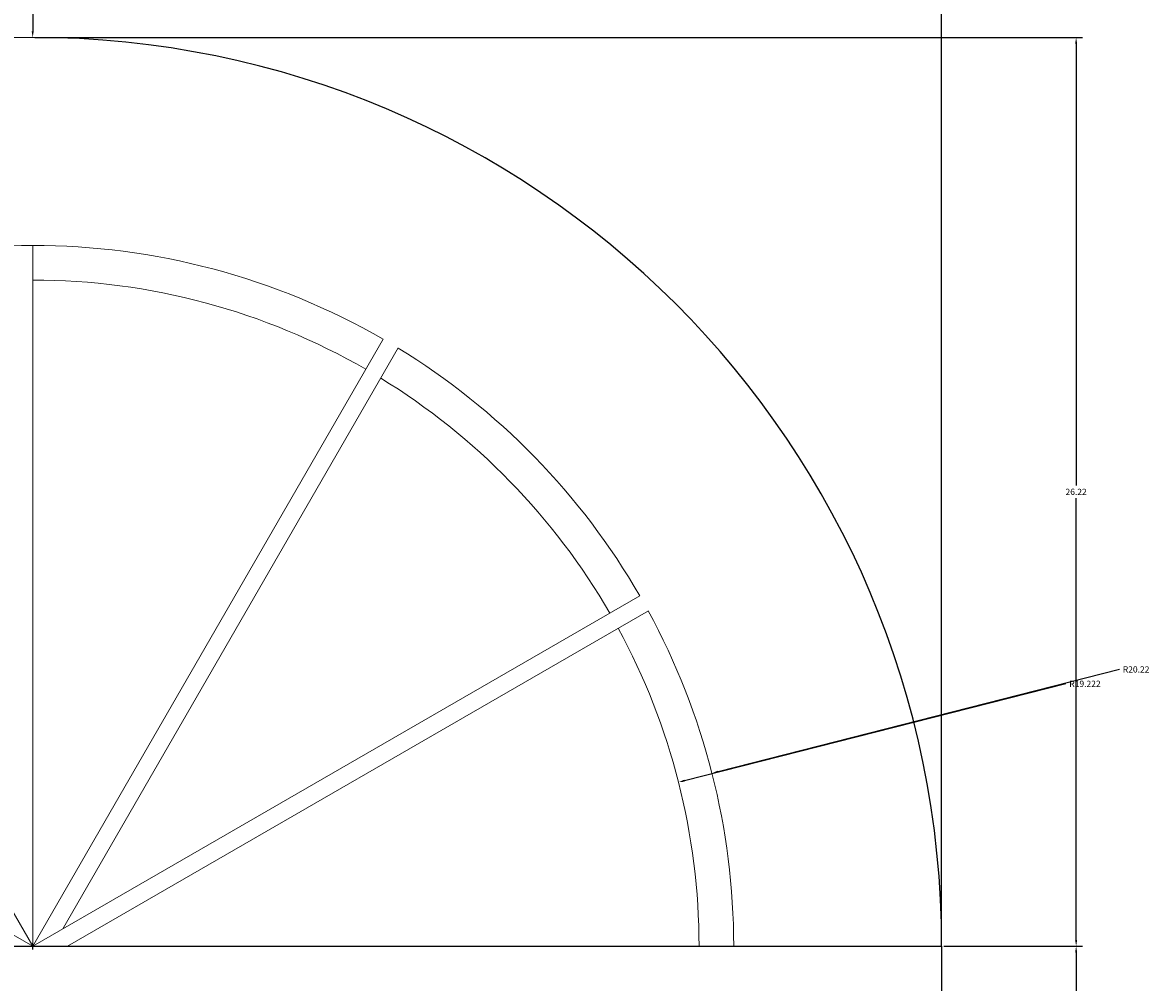
# Model space of a CAD drawing. Units: inches. Extents: x 12532.3 to 12594.9, y 6967.5 to 7063.
# Tile 8 of 9: x 12562.4 to 12594.9, y 7019.9 to 7047.6. Entities that reach past the tile are written whole.
import ezdxf

# ---------------------------------------------------------------- set-up
doc = ezdxf.new("R2010")
doc.units = ezdxf.units.IN
doc.header["$MEASUREMENT"] = 0
doc.header["$PDMODE"] = 98
for name, color, linetype, lineweight in [('A-ANNO-DIMS', 2, 'Continuous', 18), ('A-DOOR', 4, 'Continuous', 25), ('A-GLAZ', 3, 'Continuous', 18)]:
    doc.layers.add(name, color=color, linetype=linetype, lineweight=lineweight)
doc.styles.get("Standard").update_dxf_attribs({"font": 'arial.ttf'})
doc.dimstyles.get("Standard").update_dxf_attribs({"dimtxt": 0.18, "dimasz": 0.18, "dimexe": 0.18, "dimexo": 0.0625, "dimgap": 0.09, "dimtad": 0, "dimtih": 1, "dimtoh": 1, "dimdec": 4, "dimzin": 0, "dimdsep": 46, "dimtxsty": 'Standard', "dimcen": 0.09, "dimadec": 0, "dimazin": 0, "dimtfac": 1, "dimtdec": 4, "dimtofl": 0, "dimtmove": 0, "dimatfit": 3, "dimfxl": 1, "dimtolj": 1, "dimtzin": 0, "dimarcsym": 0})

# ---------------------------------------------------------------- blocks, each defined once
blk = doc.blocks.new('*D31')
at = {"layer": 'A-ANNO-DIMS', "color": 0, "lineweight": -2, "transparency": 16777216}
for p, q in [((12536.45, 7020.991), (12536.45, 7051.211)), ((12536.63, 7051.031), (12562.279, 7051.031)), ((12588.714, 7051.031), (12563.065, 7051.031)), ((12588.894, 7020.991), (12588.894, 7051.211))]:
    blk.add_line(p, q, dxfattribs=at)
at = {"layer": 'A-ANNO-DIMS', "color": 0, "transparency": 16777216}
for points in [[(12536.63, 7051.061), (12536.63, 7051.001), (12536.45, 7051.031)], [(12588.714, 7051.061), (12588.714, 7051.001), (12588.894, 7051.031)]]:
    blk.add_solid(points, dxfattribs=at)
at = {"layer": 'Defpoints', "color": 0, "transparency": 16777216}
for p in [(12588.894, 7051.031), (12536.45, 7020.929), (12588.894, 7020.929)]:
    blk.add_point(p, dxfattribs=at)
at = {"layer": 'A-ANNO-DIMS', "color": 0, "transparency": 16777216, "insert": (12562.672, 7051.031), "char_height": 0.18, "attachment_point": 5}
blk.add_mtext('\\A1;52.44', dxfattribs=at)
blk = doc.blocks.new('*D32')
at = {"layer": 'A-ANNO-DIMS', "color": 0, "lineweight": -2, "transparency": 16777216}
for p, q in [((12588.956, 7020.929), (12592.954, 7020.929)), ((12592.774, 7020.749), (12592.774, 6996.445)), ((12592.774, 6971.777), (12592.774, 6996.081)), ((12588.956, 6971.597), (12592.954, 6971.597))]:
    blk.add_line(p, q, dxfattribs=at)
at = {"layer": 'A-ANNO-DIMS', "color": 0, "transparency": 16777216}
for points in [[(12592.744, 7020.749), (12592.804, 7020.749), (12592.774, 7020.929)], [(12592.744, 6971.777), (12592.804, 6971.777), (12592.774, 6971.597)]]:
    blk.add_solid(points, dxfattribs=at)
at = {"layer": 'Defpoints', "color": 0, "transparency": 16777216}
for p in [(12588.894, 7020.929), (12592.774, 7020.929), (12588.894, 6971.597)]:
    blk.add_point(p, dxfattribs=at)
at = {"layer": 'A-ANNO-DIMS', "color": 0, "transparency": 16777216, "insert": (12592.774, 6996.263), "char_height": 0.18, "attachment_point": 5}
blk.add_mtext('\\A1;49.33', dxfattribs=at)
blk = doc.blocks.new('*D33')
at = {"layer": 'A-ANNO-DIMS', "color": 0, "lineweight": -2, "transparency": 16777216}
for p, q in [((12562.735, 7047.151), (12592.954, 7047.151)), ((12592.774, 7046.971), (12592.774, 7034.222)), ((12592.774, 7021.109), (12592.774, 7033.858)), ((12588.956, 7020.929), (12592.954, 7020.929))]:
    blk.add_line(p, q, dxfattribs=at)
at = {"layer": 'A-ANNO-DIMS', "color": 0, "transparency": 16777216}
for points in [[(12592.744, 7046.971), (12592.804, 7046.971), (12592.774, 7047.151)], [(12592.744, 7021.109), (12592.804, 7021.109), (12592.774, 7020.929)]]:
    blk.add_solid(points, dxfattribs=at)
at = {"layer": 'Defpoints', "color": 0, "transparency": 16777216}
for p in [(12562.672, 7047.151), (12592.774, 7047.151), (12588.894, 7020.929)]:
    blk.add_point(p, dxfattribs=at)
at = {"layer": 'A-ANNO-DIMS', "color": 0, "transparency": 16777216, "insert": (12592.774, 7034.04), "char_height": 0.18, "attachment_point": 5}
blk.add_mtext('\\A1;26.22', dxfattribs=at)
blk = doc.blocks.new('*D62')
at = {"layer": 'A-ANNO-DIMS', "color": 0, "lineweight": -2, "transparency": 16777216}
for p, q in [((12562.489, 7062.884), (12562.669, 7062.884)), ((12562.669, 7062.884), (12562.67, 7047.331)), ((12562.672, 7020.839), (12562.672, 7021.019)), ((12562.582, 7020.929), (12562.762, 7020.929))]:
    blk.add_line(p, q, dxfattribs=at)
at = {"layer": 'A-ANNO-DIMS', "color": 0, "transparency": 16777216}
blk.add_solid([(12562.7, 7047.331), (12562.64, 7047.331), (12562.67, 7047.151)], dxfattribs=at)
at = {"layer": 'Defpoints', "color": 0, "transparency": 16777216}
for p in [(12562.67, 7047.151), (12562.672, 7020.929)]:
    blk.add_point(p, dxfattribs=at)
at = {"layer": 'A-ANNO-DIMS', "color": 0, "transparency": 16777216, "insert": (12562.01, 7062.884), "char_height": 0.18, "attachment_point": 5}
blk.add_mtext('\\A1;R26.22', dxfattribs=at)
blk = doc.blocks.new('*D63')
at = {"layer": 'A-ANNO-DIMS', "color": 0, "lineweight": -2, "transparency": 16777216}
for p, q in [((12594.026, 7028.916), (12582.443, 7025.965)), ((12562.672, 7020.839), (12562.672, 7021.019)), ((12562.582, 7020.929), (12562.762, 7020.929))]:
    blk.add_line(p, q, dxfattribs=at)
at = {"layer": 'A-ANNO-DIMS', "color": 0, "transparency": 16777216}
blk.add_solid([(12582.435, 7025.995), (12582.45, 7025.936), (12582.268, 7025.921)], dxfattribs=at)
at = {"layer": 'Defpoints', "color": 0, "transparency": 16777216}
for p in [(12582.268, 7025.921), (12562.672, 7020.929)]:
    blk.add_point(p, dxfattribs=at)
at = {"layer": 'A-ANNO-DIMS', "color": 0, "transparency": 16777216, "insert": (12594.505, 7028.916), "char_height": 0.18, "attachment_point": 5}
blk.add_mtext('\\A1;R20.22', dxfattribs=at)
blk = doc.blocks.new('*D64')
at = {"layer": 'A-ANNO-DIMS', "color": 0, "lineweight": -2, "transparency": 16777216}
for p, q in [((12592.48, 7028.502), (12581.477, 7025.706)), ((12562.672, 7020.839), (12562.672, 7021.019)), ((12562.582, 7020.929), (12562.762, 7020.929))]:
    blk.add_line(p, q, dxfattribs=at)
at = {"layer": 'A-ANNO-DIMS', "color": 0, "transparency": 16777216}
blk.add_solid([(12581.469, 7025.735), (12581.484, 7025.677), (12581.302, 7025.662)], dxfattribs=at)
at = {"layer": 'Defpoints', "color": 0, "transparency": 16777216}
for p in [(12581.302, 7025.662), (12562.672, 7020.929)]:
    blk.add_point(p, dxfattribs=at)
at = {"layer": 'A-ANNO-DIMS', "color": 0, "transparency": 16777216, "insert": (12593.029, 7028.502), "char_height": 0.18, "attachment_point": 5}
blk.add_mtext('\\A1;R19.222', dxfattribs=at)

msp = doc.modelspace()

# ---------------------------------------------------------------- linework, layer by layer
at = {"layer": 'A-DOOR'}
msp.add_lwpolyline([(12536.4501, 7020.9287), (12588.894, 7020.9287), (12588.894, 6971.5968), (12536.4501, 6971.5968)], close=True, dxfattribs=at)
msp.add_arc((12562.6721, 7020.9287), 26.2219, 0, 180, dxfattribs=at)
at = {"layer": 'A-GLAZ'}
for p, q in [((12562.6721, 7040.1506), (12562.6721, 7041.1506)), ((12562.6721, 7020.9287), (12562.6721, 7040.1506)), ((12562.6721, 7020.9287), (12552.5611, 7038.4414)), ((12562.6721, 7020.9287), (12572.783, 7038.4414)), ((12563.5381, 7021.4287), (12573.216, 7038.1914)), ((12562.6721, 7020.9287), (12545.1594, 7031.0397)), ((12562.6721, 7020.9287), (12580.1848, 7031.0397)), ((12563.6721, 7020.9287), (12580.4348, 7030.6067))]:
    msp.add_line(p, q, dxfattribs=at)
for radius, start, end in [(20.2219, 60, 120), (19.2219, 60, 90), (20.2219, 30, 58.58318), (19.2219, 30, 58.50946), (20.2219, 0, 28.58318), (19.2219, 0, 28.50946)]:
    msp.add_arc((12562.6721, 7020.9287), radius, start, end, dxfattribs=at)

# ---------------------------------------------------------------- dimensions: what is measured, and where the dimension line sits
at = {"layer": 'A-ANNO-DIMS'}
for mpoint, override, picture, middle in [((12562.67, 7047.1506), {"dimdec": 2, "dimlfac": 1, "dimrnd": 0, "dimzin": 0, "dimdsep": 46, "dimlunit": 2}, '*D62', (12562.0098, 7062.8838)), ((12582.2681, 7025.921), {"dimdec": 2, "dimlfac": 1, "dimrnd": 0, "dimzin": 0, "dimdsep": 46, "dimlunit": 2}, '*D63', (12594.0257, 7028.9164)), ((12581.3021, 7025.662), {"dimdec": 3, "dimlfac": 1, "dimrnd": 0, "dimzin": 0, "dimdsep": 46, "dimlunit": 2}, '*D64', (12592.4801, 7028.502))]:
    dim = msp.add_radius_dim(center=(12562.6721, 7020.9287), mpoint=mpoint, dimstyle='Standard', override=override, dxfattribs=at)
    dim.commit()
    dim.dimension.update_dxf_attribs({"geometry": picture, "text_midpoint": middle, "dimtype": 164})
dim = msp.add_linear_dim(base=(12588.894, 7051.0306), p1=(12536.4501, 7020.9287), p2=(12588.894, 7020.9287), dimstyle='Standard', override={"dimdec": 2, "dimlfac": 1, "dimrnd": 0, "dimzin": 0, "dimdsep": 46, "dimlunit": 2}, dxfattribs=at)
dim.commit()
dim.dimension.update_dxf_attribs({"geometry": '*D31', "text_midpoint": (12562.6721, 7051.0306)})
for base, p1, p2, picture, middle in [((12592.774, 7047.1506), (12588.894, 7020.9287), (12562.6721, 7047.1506), '*D33', (12592.774, 7034.0397)), ((12592.774, 7020.9287), (12588.894, 6971.5968), (12588.894, 7020.9287), '*D32', (12592.774, 6996.2627))]:
    dim = msp.add_linear_dim(base=base, p1=p1, p2=p2, angle=90, dimstyle='Standard', override={"dimdec": 2, "dimlfac": 1, "dimrnd": 0, "dimzin": 0, "dimdsep": 46, "dimlunit": 2}, dxfattribs=at)
    dim.commit()
    dim.dimension.update_dxf_attribs({"geometry": picture, "text_midpoint": middle})

doc.saveas('drawing.dxf')
